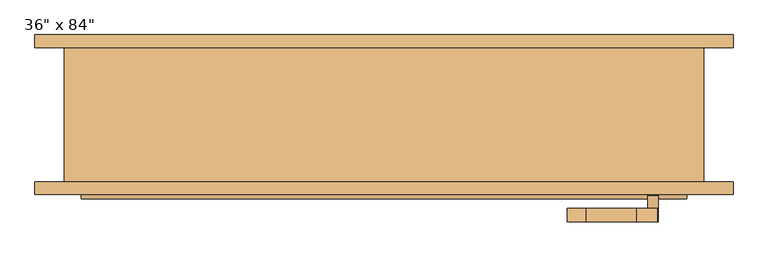
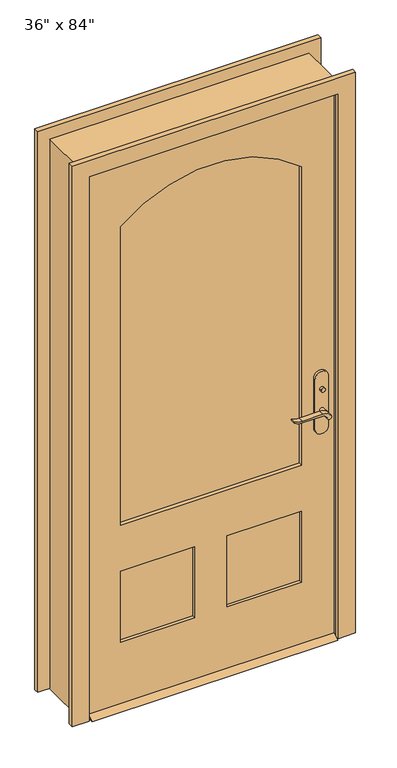
"""IFC4 building model written with IfcOpenShell, lengths in millimetres: door geometry."""

from ifc_helpers import new_model, si_unit, point, frame, frame_2d, origin, place, context, project, spatial, polyline, circle_curve, trimmed, segment, composite_curve, outline, extrude, faceted_brep, source, transform, mapped, element, save


def door_9fdf8246(model_context):
    return source(origin(), model_context, "Body", "SolidModel", [
        extrude(outline(polyline([(-63.5, 12.7), (-38.1, 0.0), (-123.825, 0.0), (-98.425, 12.7), (-63.5, 12.7)])), frame((-457.2, 0.0, 0.0), z_axis=(1.0, 0.0, 0.0), x_axis=(0.0, 1.0, 0.0)), (0.0, 0.0, 1.0), 914.4),
        extrude(outline(polyline([(411.4, -43.5), (411.4, -53.5), (401.4, -53.5), (401.4, -43.5), (411.4, -43.5)])), frame((0.0, 0.0, 981.9), z_axis=(0.0, 0.0, 1.0), x_axis=(1.0, 0.0, 0.0)), (0.0, 0.0, 1.0), 30.0),
        extrude(outline(composite_curve([segment(trimmed(circle_curve(frame_2d((996.9, 406.4)), 8.0), [point((996.9, 398.4))], [point((996.9, 414.4))], False, "CARTESIAN"), True, "CONTINUOUS"), segment(trimmed(circle_curve(frame_2d((996.9, 406.4)), 8.0), [point((996.9, 414.4))], [point((996.9, 398.4))], False, "CARTESIAN"), True, "CONTINUOUS")], self_intersect=False)), frame((0.0, -118.425, 0.0), z_axis=(0.0, 1.0, 0.0), x_axis=(0.0, 0.0, 1.0)), (0.0, 0.0, 1.0), 10.0),
        extrude(outline(composite_curve([segment(trimmed(circle_curve(frame_2d((897.1555521, 382.7324871)), 37.2832219), [point((919.0523287, 412.9081363))], [point((934.4, 381.0325667))], False, "CARTESIAN"), True, "CONTINUOUS"), segment(polyline([(934.4, 381.0325667), (934.4, 304.7564091)]), True, "CONTINUOUS"), segment(trimmed(circle_curve(frame_2d((1017.6850638, 304.8227909)), 83.2850902), [point((934.4, 304.7564091))], [point((939.4, 276.4))], True, "CARTESIAN"), True, "CONTINUOUS"), segment(polyline([(939.4, 276.4), (936.6135558, 276.4)]), True, "CONTINUOUS"), segment(trimmed(circle_curve(frame_2d((986.6709207, 308.3396612)), 59.3791355), [point((936.6135558, 276.4))], [point((927.4, 304.7564091))], False, "CARTESIAN"), True, "CONTINUOUS"), segment(polyline([(927.4, 304.7564091), (927.4, 381.0138099)]), True, "CONTINUOUS"), segment(trimmed(circle_curve(frame_2d((909.2738613, 381.0138099)), 18.1261387), [point((927.4, 381.0138099))], [point((914.4, 398.4))], True, "CARTESIAN"), True, "CONTINUOUS"), segment(trimmed(circle_curve(frame_2d((914.4, 406.4)), 8.0), [point((914.4, 398.4))], [point((919.0523287, 412.9081363))], False, "CARTESIAN"), True, "CONTINUOUS")], self_intersect=False)), frame((0.0, -23.5, 0.0), z_axis=(0.0, 1.0, 0.0), x_axis=(0.0, 0.0, 1.0)), (0.0, 0.0, 1.0), 20.0),
        extrude(outline(composite_curve([segment(trimmed(circle_curve(frame_2d((914.4, 406.4)), 8.0), [point((914.3999903, 398.4))], [point((919.0523287, 412.9081363))], False, "CARTESIAN"), True, "CONTINUOUS"), segment(trimmed(circle_curve(frame_2d((897.1555521, 382.7324871)), 37.2832219), [point((919.0523287, 412.9081363))], [point((934.4, 381.0325667))], False, "CARTESIAN"), True, "CONTINUOUS"), segment(polyline([(934.4, 381.0325667), (934.4, 304.7564091)]), True, "CONTINUOUS"), segment(trimmed(circle_curve(frame_2d((1017.6850638, 304.8227909)), 83.2850902), [point((934.4, 304.7564091))], [point((939.4, 276.4))], True, "CARTESIAN"), True, "CONTINUOUS"), segment(polyline([(939.4, 276.4), (936.6135558, 276.4)]), True, "CONTINUOUS"), segment(trimmed(circle_curve(frame_2d((986.6709207, 308.3396612)), 59.3791355), [point((936.6135558, 276.4))], [point((927.4, 304.7564091))], False, "CARTESIAN"), True, "CONTINUOUS"), segment(polyline([(927.4, 304.7564091), (927.4, 381.0138122)]), True, "CONTINUOUS"), segment(trimmed(circle_curve(frame_2d((909.2738682, 381.0138122)), 18.1261318), [point((927.4, 381.0138122))], [point((914.3999903, 398.4))], True, "CARTESIAN"), True, "CONTINUOUS")], self_intersect=False)), frame((0.0, -158.425, 0.0), z_axis=(0.0, 1.0, 0.0), x_axis=(0.0, 0.0, 1.0)), (0.0, 0.0, 1.0), 20.0),
        extrude(outline(composite_curve([segment(trimmed(circle_curve(frame_2d((914.4, 406.4)), 8.0), [point((914.4, 398.4))], [point((914.4, 414.4))], False, "CARTESIAN"), True, "CONTINUOUS"), segment(trimmed(circle_curve(frame_2d((914.4, 406.4)), 8.0), [point((914.4, 414.4))], [point((914.4, 398.4))], False, "CARTESIAN"), True, "CONTINUOUS")], self_intersect=False)), frame((0.0, -53.5, 0.0), z_axis=(0.0, 1.0, 0.0), x_axis=(0.0, 0.0, 1.0)), (0.0, 0.0, 1.0), 30.0),
        extrude(outline(composite_curve([segment(trimmed(circle_curve(frame_2d((914.4, 406.4)), 8.0), [point((914.4, 398.4))], [point((914.4, 414.4))], False, "CARTESIAN"), True, "CONTINUOUS"), segment(trimmed(circle_curve(frame_2d((914.4, 406.4)), 8.0), [point((914.4, 414.4))], [point((914.4, 398.4))], False, "CARTESIAN"), True, "CONTINUOUS")], self_intersect=False)), frame((0.0, -138.425, 0.0), z_axis=(0.0, 1.0, 0.0), x_axis=(0.0, 0.0, 1.0)), (0.0, 0.0, 1.0), 30.0),
        extrude(outline(composite_curve([segment(polyline([(844.4, 431.4), (1039.4, 431.4)]), True, "CONTINUOUS"), segment(trimmed(circle_curve(frame_2d((1039.4, 406.4)), 25.0), [point((1039.4, 431.4))], [point((1039.4, 381.4))], False, "CARTESIAN"), True, "CONTINUOUS"), segment(polyline([(1039.4, 381.4), (844.4, 381.4)]), True, "CONTINUOUS"), segment(trimmed(circle_curve(frame_2d((844.4, 406.4)), 25.0), [point((844.4, 381.4))], [point((844.4, 431.4))], False, "CARTESIAN"), True, "CONTINUOUS")], self_intersect=False)), frame((0.0, -63.5, 0.0), z_axis=(0.0, 1.0, 0.0), x_axis=(0.0, 0.0, 1.0)), (0.0, 0.0, 1.0), 10.0),
        extrude(outline(composite_curve([segment(polyline([(844.4, 431.4), (1039.4, 431.4)]), True, "CONTINUOUS"), segment(trimmed(circle_curve(frame_2d((1039.4, 406.4)), 25.0), [point((1039.4, 431.4))], [point((1039.4, 381.4))], False, "CARTESIAN"), True, "CONTINUOUS"), segment(polyline([(1039.4, 381.4), (844.4, 381.4)]), True, "CONTINUOUS"), segment(trimmed(circle_curve(frame_2d((844.4, 406.4)), 25.0), [point((844.4, 381.4))], [point((844.4, 431.4))], False, "CARTESIAN"), True, "CONTINUOUS")], self_intersect=False)), frame((0.0, -108.425, 0.0), z_axis=(0.0, 1.0, 0.0), x_axis=(0.0, 0.0, 1.0)), (0.0, 0.0, 1.0), 10.0),
        extrude(outline(polyline([(2133.6, -457.2), (12.7, -457.2), (12.7, 457.2), (2133.6, 457.2), (2133.6, -457.2)]), holes=[composite_curve([segment(polyline([(714.375, -336.55), (1885.95, -336.55)]), True, "CONTINUOUS"), segment(trimmed(circle_curve(frame_2d((1503.52125, 0.0)), 509.42875), [point((1885.95, -336.55))], [point((1885.95, 336.55))], True, "CARTESIAN"), True, "CONTINUOUS"), segment(polyline([(1885.95, 336.55), (714.375, 336.55), (714.375, -336.55)]), True, "CONTINUOUS")], self_intersect=False), polyline([(533.4, -60.325), (254.0, -60.325), (254.0, -336.55), (533.4, -336.55), (533.4, -60.325)]), polyline([(533.4, 336.55), (254.0, 336.55), (254.0, 60.325), (533.4, 60.325), (533.4, 336.55)])]), frame((0.0, -98.425, 0.0), z_axis=(0.0, 1.0, 0.0), x_axis=(0.0, 0.0, 1.0)), (0.0, 0.0, 1.0), 34.925),
        faceted_brep([(482.6, -98.425, 0.0), (457.2, -98.425, 0.0), (457.2, -63.5, 0.0), (444.5, -63.5, 0.0), (444.5, -28.575, 0.0), (457.2, -28.575, 0.0), (457.2, 104.775, 0.0), (482.6, 104.775, 0.0), (482.6, 104.775, 2159.0), (482.6, -98.425, 2159.0), (457.2, 104.775, 2133.6), (-457.2, 104.775, 2133.6), (-457.2, 104.775, 0.0), (-482.6, 104.775, 0.0), (-482.6, 104.775, 2159.0), (457.2, -28.575, 2133.6), (444.5, -28.575, 2120.9), (-444.5, -28.575, 2120.9), (-444.5, -28.575, 0.0), (-457.2, -28.575, 0.0), (-457.2, -28.575, 2133.6), (444.5, -63.5, 2120.9), (457.2, -63.5, 2133.6), (-457.2, -63.5, 2133.6), (-457.2, -63.5, 0.0), (-444.5, -63.5, 0.0), (-444.5, -63.5, 2120.9), (457.2, -98.425, 2133.6), (-482.6, -98.425, 2159.0), (-482.6, -98.425, 0.0), (-457.2, -98.425, 0.0), (-457.2, -98.425, 2133.6)], [[[0, 1, 2, 3, 4, 5, 6, 7]], [[7, 8, 9, 0]], [[6, 10, 11, 12, 13, 14, 8, 7]], [[5, 15, 10, 6]], [[4, 16, 17, 18, 19, 20, 15, 5]], [[3, 21, 16, 4]], [[2, 22, 23, 24, 25, 26, 21, 3]], [[1, 27, 22, 2]], [[0, 9, 28, 29, 30, 31, 27, 1]], [[8, 14, 28, 9]], [[15, 20, 11, 10]], [[21, 26, 17, 16]], [[27, 31, 23, 22]], [[29, 13, 12, 19, 18, 25, 24, 30]], [[14, 13, 29, 28]], [[20, 19, 12, 11]], [[26, 25, 18, 17]], [[31, 30, 24, 23]]]),
        extrude(outline(polyline([(-60.325, -75.1416667), (-60.325, -86.7833333), (-336.55, -86.7833333), (-336.55, -75.1416667), (-60.325, -75.1416667)])), frame((0.0, 0.0, 254.0), z_axis=(0.0, 0.0, 1.0), x_axis=(1.0, 0.0, 0.0)), (0.0, 0.0, 1.0), 279.4),
        extrude(outline(polyline([(336.55, -75.1416667), (336.55, -86.7833333), (60.325, -86.7833333), (60.325, -75.1416667), (336.55, -75.1416667)])), frame((0.0, 0.0, 254.0), z_axis=(0.0, 0.0, 1.0), x_axis=(1.0, 0.0, 0.0)), (0.0, 0.0, 1.0), 279.4),
        extrude(outline(composite_curve([segment(polyline([(714.375, -336.55), (714.375, 336.55), (1885.95, 336.55)]), True, "CONTINUOUS"), segment(trimmed(circle_curve(frame_2d((1503.52125, 0.0)), 509.42875), [point((1885.95, 336.55))], [point((1885.95, -336.55))], False, "CARTESIAN"), True, "CONTINUOUS"), segment(polyline([(1885.95, -336.55), (714.375, -336.55)]), True, "CONTINUOUS")], self_intersect=False)), frame((0.0, -84.455, 0.0), z_axis=(0.0, 1.0, 0.0), x_axis=(0.0, 0.0, 1.0)), (0.0, 0.0, 1.0), 6.985),
        extrude(outline(polyline([(0.0, -463.55), (2139.95, -463.55), (2139.95, 463.55), (0.0, 463.55), (0.0, 527.05), (2203.45, 527.05), (2203.45, -527.05), (0.0, -527.05), (0.0, -463.55)])), frame((0.0, 104.775, 0.0), z_axis=(0.0, 1.0, 0.0), x_axis=(0.0, 0.0, 1.0)), (0.0, 0.0, 1.0), 19.05),
        extrude(outline(polyline([(0.0, -463.55), (2139.95, -463.55), (2139.95, 463.55), (0.0, 463.55), (0.0, 527.05), (2203.45, 527.05), (2203.45, -527.05), (0.0, -527.05), (0.0, -463.55)])), frame((0.0, -117.475, 0.0), z_axis=(0.0, 1.0, 0.0), x_axis=(0.0, 0.0, 1.0)), (0.0, 0.0, 1.0), 19.05),
    ])


if __name__ == "__main__":
    model = new_model("IFC4")
    model_context = context("Model", 3, world=origin())
    ifc_project = project(units=[si_unit("LENGTHUNIT", "METRE", prefix="MILLI")], contexts=[model_context])
    site = spatial("IfcSite", under=ifc_project)
    building = spatial("IfcBuilding", under=site)
    placement = place(None, origin())
    door_shape = door_9fdf8246(model_context)
    element("IfcDoor", 1, ObjectType="36\" x 84\"", at=placement, inside=building, context=model_context, shape_type="MappedRepresentation", body=[
        mapped(door_shape, transform((0.0, 0.0, 0.0), x_axis=(1.0, 0.0, 0.0), y_axis=(0.0, 1.0, 0.0), z_axis=(0.0, 0.0, 1.0))),
    ])
    save(model, "model.ifc")

# Revit data of these elements
# Type "36\" x 84\""
#   Type Mark = "11"
#   Assembly Code = "B2030100"
#   Analytic Construction = "French door, wood frame with single glass"
#   Threshold Offset [instance default] = 0' - 0 1/2"
#   Thickness = 0' - 1 3/8"
#   Thermal Resistance (R) = 1.0696 (h·ft²·°F)/BTU
#   Swing Angle [instance default] = 90.00°
#   Stiles = 0' - 4 3/4"
#   Rough Width = 3' - 2"
#   Rough Height = 7' - 1"
#   Radius = 1' - 8.05625"
#   Lock Rail = 0' - 7 1/8"
#   Height = 7' - 0"
#   Width = 3' - 0"
#   Heat Transfer Coefficient (U) = 0.9350 BTU/(h·ft²·°F)
#   Door Offset [instance default] = 0' - 0"
#   Bottom Rail = 0' - 9 1/2"
#   Threshold [instance default] = yes
#   Function = 1
#   Exterior Trim [instance default] = yes
#   Trim Material = Cherry
#   Threshold Material = Cherry
#   Panel Material = Cherry
#   Glazing = Glass
#   Frame Material = Cherry
#   Door Handle Material = Aluminum
#   Visual Light Transmittance = 0
#   Solar Heat Gain Coefficient = 0
#   Wall Closure = (empty or 0)
#   Construction Type = (empty or 0)
# Element 1 (IfcDoor, "36\" x 84\"")
#   Materials on its faces: "Cherry", "Aluminum", "Glass"
# Materials
#   "Cherry": class "Wood", colour RGB 226 177 128, transparency 0, Description = "Prunus Serotina", Cost = 0
#   "Glass": class "Glass", colour RGB 0 128 192, transparency 0.75, Description = "Soda Lime Glass", Cost = 0
#   "Aluminum": class "Metal", colour RGB 247 247 247, transparency 0, Description = "Aluminum 6061", Cost = 0
